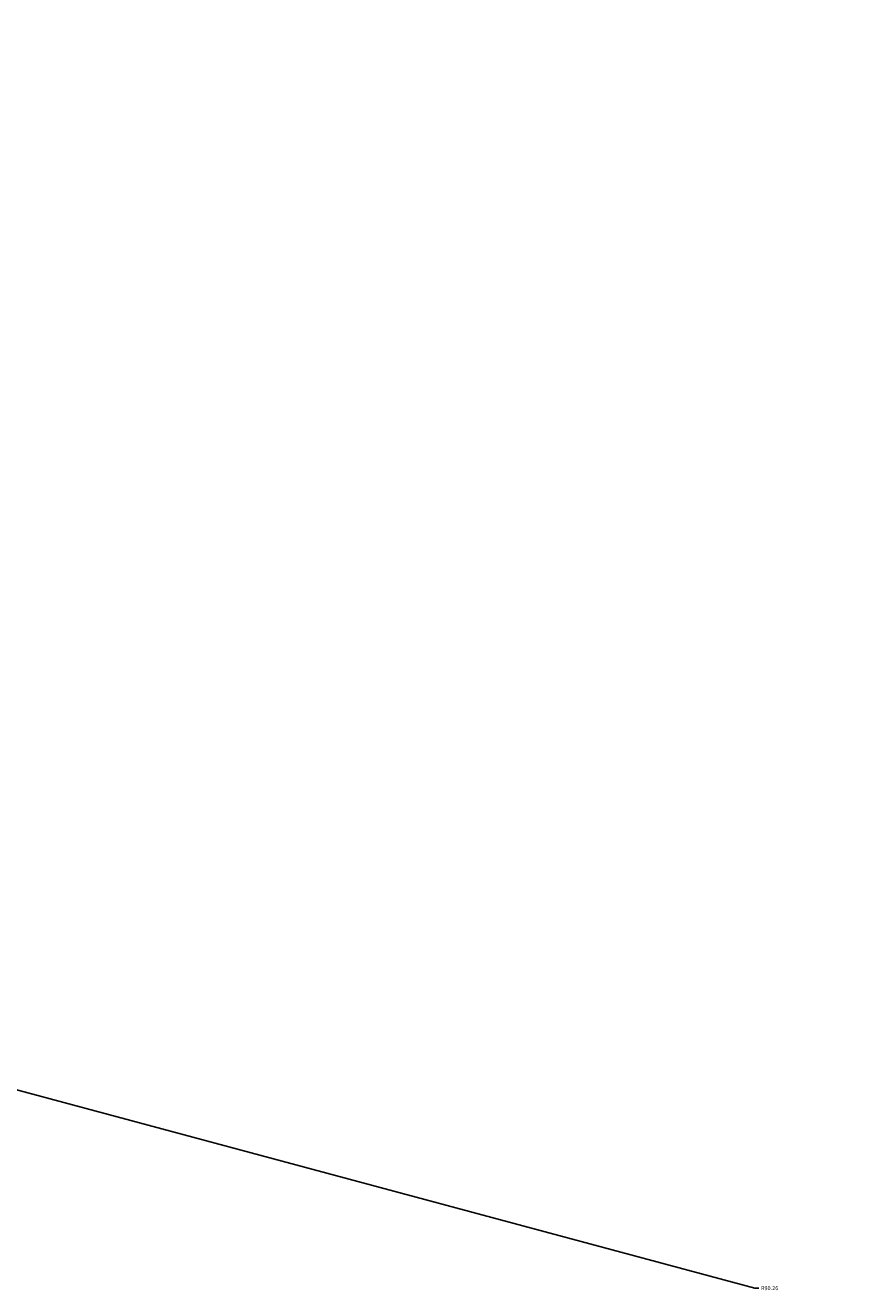
# Model space of a CAD drawing. Units: inches. Extents: x -12 to 334, y -10 to 186.
# Tile 74 of 77: x 297 to 334, y 54 to 111. Entities that reach past the tile are written whole.
import ezdxf

# ---------------------------------------------------------------- set-up
doc = ezdxf.new("R2010")
doc.units = ezdxf.units.IN
doc.header["$MEASUREMENT"] = 0
doc.layers.add('M-DIMS', color=2, linetype='Continuous', lineweight=18)
doc.styles.get("Standard").update_dxf_attribs({"font": 'arial.ttf'})
doc.dimstyles.get("Standard").update_dxf_attribs({"dimtxt": 0.18, "dimasz": 0.18, "dimexe": 0.18, "dimexo": 0.0625, "dimgap": 0.09, "dimtad": 0, "dimtih": 1, "dimtoh": 1, "dimdec": 4, "dimzin": 0, "dimdsep": 46, "dimtxsty": 'Standard', "dimcen": 0.09, "dimadec": 0, "dimazin": 0, "dimtfac": 1, "dimtdec": 4, "dimtofl": 0, "dimtmove": 0, "dimatfit": 3, "dimfxl": 1, "dimtolj": 1, "dimtzin": 0, "dimarcsym": 0})

# ---------------------------------------------------------------- blocks, each defined once
blk = doc.blocks.new('*D40')
at = {"layer": 'Defpoints', "color": 0, "transparency": 16777216}
for p in [(278.229, 116.208), (187.394, 91.899)]:
    blk.add_point(p, dxfattribs=at)
at = {"layer": 'M-DIMS', "color": 0, "lineweight": -2, "transparency": 16777216}
for p, q in [((332.73, 130.793), (278.403, 116.254)), ((187.304, 91.899), (187.484, 91.899)), ((187.394, 91.809), (187.394, 91.989))]:
    blk.add_line(p, q, dxfattribs=at)
at = {"layer": 'M-DIMS', "color": 0, "transparency": 16777216}
blk.add_solid([(278.395, 116.283), (278.411, 116.225), (278.229, 116.208)], dxfattribs=at)
at = {"layer": 'M-DIMS', "color": 0, "transparency": 16777216, "insert": (333.21, 130.793), "char_height": 0.18, "attachment_point": 5}
blk.add_mtext('\\A1;R94.03', dxfattribs=at)
blk = doc.blocks.new('*D41')
at = {"layer": 'Defpoints', "color": 0, "transparency": 16777216}
for p in [(190.169, 91.899), (277.343, 68.515)]:
    blk.add_point(p, dxfattribs=at)
at = {"layer": 'M-DIMS', "color": 0, "lineweight": -2, "transparency": 16777216}
for p, q in [((190.079, 91.899), (190.259, 91.899)), ((190.169, 91.809), (190.169, 91.989)), ((329.648, 54.485), (277.517, 68.469)), ((329.828, 54.485), (329.648, 54.485))]:
    blk.add_line(p, q, dxfattribs=at)
at = {"layer": 'M-DIMS', "color": 0, "transparency": 16777216}
blk.add_solid([(277.525, 68.498), (277.509, 68.44), (277.343, 68.515)], dxfattribs=at)
at = {"layer": 'M-DIMS', "color": 0, "transparency": 16777216, "insert": (330.307, 54.485), "char_height": 0.18, "attachment_point": 5}
blk.add_mtext('\\A1;R90.26', dxfattribs=at)

msp = doc.modelspace()

# ---------------------------------------------------------------- dimensions: what is measured, and where the dimension line sits
at = {"layer": 'M-DIMS'}
for center, mpoint, picture, middle in [((187.3936, 91.8988), (278.2291, 116.2078), '*D40', (332.7304, 130.7932)), ((190.1689, 91.8988), (277.3431, 68.5153), '*D41', (330.3074, 54.4851))]:
    dim = msp.add_radius_dim(center=center, mpoint=mpoint, dimstyle='Standard', override={"dimdec": 2, "dimlfac": 1, "dimrnd": 0, "dimzin": 0, "dimdsep": 46, "dimlunit": 2}, dxfattribs=at)
    dim.commit()
    dim.dimension.update_dxf_attribs({"geometry": picture, "text_midpoint": middle, "dimtype": 164})

doc.saveas('drawing.dxf')
